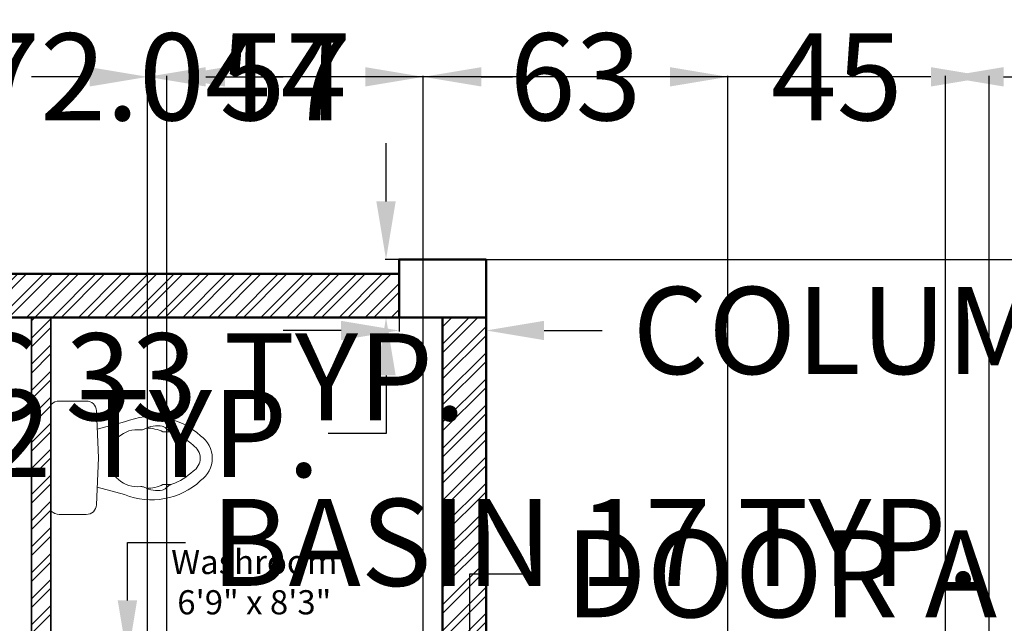
# Model space of a CAD drawing. Units: inches. Extents: x -90 to 536, y -553 to 299.
# Tile 26 of 27: x 207 to 410, y 174 to 299. Entities that reach past the tile are written whole.
import ezdxf

# ---------------------------------------------------------------- set-up
doc = ezdxf.new("R2010")
doc.units = ezdxf.units.IN
for name, color, linetype, lineweight in [('A-ANNO-DIMS', 2, 'Continuous', 18), ('A-AREA-IDEN', 7, 'Continuous', 18), ('A-COLS', 7, 'Continuous', 50), ('A-FLOR-FIXT', 8, 'Continuous', 18), ('A-WALL-PATT', 252, 'Continuous', 13), ('Inner Wall', 5, 'Continuous', 35), ('Outer Wall', 1, 'Continuous', 50)]:
    doc.layers.add(name, color=color, linetype=linetype, lineweight=lineweight)
doc.styles.get("Standard").update_dxf_attribs({"font": 'arial.ttf'})
doc.dimstyles.get("Standard").update_dxf_attribs({"dimtxt": 18, "dimasz": 12, "dimexe": 0.18, "dimexo": 0.0625, "dimgap": 0.09, "dimtad": 0, "dimtih": 1, "dimtoh": 1, "dimdec": 0, "dimzin": 0, "dimdsep": 46, "dimlunit": 3, "dimtxsty": 'Standard', "dimcen": 0.09, "dimadec": 0, "dimazin": 0, "dimtfac": 1, "dimtdec": 0, "dimtofl": 0, "dimtmove": 0, "dimatfit": 3, "dimfxl": 1, "dimtolj": 1, "dimtzin": 0, "dimarcsym": 0})

# ---------------------------------------------------------------- blocks, each defined once
blk = doc.blocks.new('A$C1308471B')
at = {"ltscale": 20}
for p, q in [((0, 0.4607), (0, 0.0186)), ((0.0354, 0.4793), (0.1495, 0.4793)), ((0.2013, 0.2397), (0.1923, 0.4384)), ((0.1957, 0.3639), (0.3109, 0.3953)), ((0.5021, 0.3528), (0.4724, 0.3528)), ((0.4982, 0.3575), (0.4822, 0.3709)), ((0.2013, 0.2397), (0.1923, 0.0409)), ((0.5021, 0.1304), (0.4724, 0.1304)), ((0.4982, 0.1257), (0.4822, 0.1123)), ((0.1959, 0.1193), (0.3109, 0.0879)), ((0.0354, 0), (0.1495, 0))]:
    blk.add_line(p, q, dxfattribs=at)
for centre, radius, start, end in [((0.006, 0.4607), 0.006, 136.5269, 180), ((0.0354, 0.4328), 0.0465, 90, 136.5269), ((0.1495, 0.4365), 0.0429, 2.5755, 90), ((0.4248, 0.1104), 0.3068, 47.4135, 111.7924), ((0.4494, 0.2636), 0.1148, 79.3968, 118.5742), ((0.4658, 0.3513), 0.0255, 50, 79.3968), ((0.3654, 0.2416), 0.1206, 83.3523, 180), ((0.3823, 0.3868), 0.0255, 263.3523, 298.5742), ((0.405, 0.2159), 0.153, 63.502, 90.4522), ((0.5146, 0.377), 0.0255, 230, 251.3881), ((0.5021, 0.3273), 0.0255, 70.3751, 90), ((0.4248, 0.1104), 0.2558, 46.612, 70.3751), ((0.5654, 0.2416), 0.116, 0, 54.7115), ((0.5654, 0.2416), 0.065, 0, 57.2974), ((0.3654, 0.2416), 0.1206, 180, 276.6477), ((0.5654, 0.2416), 0.065, 302.7026, 0), ((0.5654, 0.2416), 0.116, 305.2885, 0), ((0.4248, 0.3728), 0.2558, 289.6249, 313.388), ((0.4248, 0.3728), 0.3068, 248.2076, 312.5865), ((0.405, 0.2673), 0.153, 269.5478, 296.498), ((0.5146, 0.1062), 0.0255, 108.6119, 130), ((0.5021, 0.1559), 0.0255, 270, 289.6249), ((0.3823, 0.0964), 0.0255, 61.4258, 96.6477), ((0.4494, 0.2196), 0.1148, 241.4258, 280.6032), ((0.4658, 0.1319), 0.0255, 280.6032, 310), ((0.006, 0.0186), 0.006, 180, 223.4731), ((0.0354, 0.0465), 0.0465, 223.4731, 270), ((0.1495, 0.0429), 0.0429, 270, 357.4245)]:
    blk.add_arc(centre, radius, start, end, dxfattribs=at)
blk = doc.blocks.new('COL-12X18')
blk.add_lwpolyline([(0, 18), (12, 18), (12, 0), (0, 0)], close=True)
blk = doc.blocks.new('*D19')
at = {"layer": 'A-ANNO-DIMS', "color": 0, "lineweight": -2, "transparency": 16777216}
for p, q in [((299.76, 172.45), (299.76, 184.45)), ((299.76, 184.45), (311.76, 184.45)), ((294.19, 172.45), (299.94, 172.45)), ((299.76, 146.95), (299.76, 160.45)), ((294.19, 134.95), (299.94, 134.95))]:
    blk.add_line(p, q, dxfattribs=at)
at = {"layer": 'A-ANNO-DIMS', "color": 0, "transparency": 16777216}
for points in [[(297.76, 160.45), (301.76, 160.45), (299.76, 172.45)], [(297.76, 146.95), (301.76, 146.95), (299.76, 134.95)]]:
    blk.add_solid(points, dxfattribs=at)
at = {"layer": 'Defpoints', "color": 0, "transparency": 16777216}
for p in [(294.13, 172.45), (299.76, 172.45), (294.13, 134.95)]:
    blk.add_point(p, dxfattribs=at)
at = {"layer": 'A-ANNO-DIMS', "color": 0, "transparency": 16777216, "insert": (408.3, 184.45), "char_height": 18, "attachment_point": 5}
blk.add_mtext('\\A1;DOOR A 38 TYP.', dxfattribs=at)
blk = doc.blocks.new('*D21')
at = {"layer": 'A-ANNO-DIMS', "color": 0, "lineweight": -2, "transparency": 16777216}
for p, q in [((122.13, 220.23), (122.13, 225.35)), ((134.13, 225.17), (143.49, 225.17)), ((155.49, 220.23), (155.49, 225.35)), ((155.49, 225.17), (167.49, 225.17))]:
    blk.add_line(p, q, dxfattribs=at)
at = {"layer": 'A-ANNO-DIMS', "color": 0, "transparency": 16777216}
for points in [[(134.13, 227.17), (134.13, 223.17), (122.13, 225.17)], [(143.49, 227.17), (143.49, 223.17), (155.49, 225.17)]]:
    blk.add_solid(points, dxfattribs=at)
at = {"layer": 'Defpoints', "color": 0, "transparency": 16777216}
for p in [(155.49, 225.17), (122.13, 220.17), (155.49, 220.17)]:
    blk.add_point(p, dxfattribs=at)
at = {"layer": 'A-ANNO-DIMS', "color": 0, "transparency": 16777216, "insert": (236.2, 225.17), "char_height": 18, "attachment_point": 5}
blk.add_mtext('\\A1;WC 33 TYP.', dxfattribs=at)
blk = doc.blocks.new('*D23')
at = {"layer": 'A-ANNO-DIMS', "color": 0, "lineweight": -2, "transparency": 16777216}
for p, q in [((285.13, 237.38), (285.13, 234.57)), ((303.13, 237.38), (303.13, 234.57)), ((273.13, 234.75), (261.13, 234.75)), ((315.13, 234.75), (327.13, 234.75))]:
    blk.add_line(p, q, dxfattribs=at)
at = {"layer": 'A-ANNO-DIMS', "color": 0, "transparency": 16777216}
for points in [[(273.13, 236.75), (273.13, 232.75), (285.13, 234.75)], [(315.13, 236.75), (315.13, 232.75), (303.13, 234.75)]]:
    blk.add_solid(points, dxfattribs=at)
at = {"layer": 'Defpoints', "color": 0, "transparency": 16777216}
for p in [(285.13, 237.45), (303.13, 237.45), (303.13, 234.75)]:
    blk.add_point(p, dxfattribs=at)
at = {"layer": 'A-ANNO-DIMS', "color": 0, "transparency": 16777216, "insert": (428.9, 234.75), "char_height": 18, "attachment_point": 5}
blk.add_mtext('\\A1;COLUMN 18 TYP.', dxfattribs=at)
blk = doc.blocks.new('*D24')
at = {"layer": 'A-ANNO-DIMS', "color": 0, "lineweight": -2, "transparency": 16777216}
for p, q in [((282.43, 261.45), (282.43, 273.45)), ((285.07, 249.45), (282.25, 249.45)), ((285.07, 237.45), (282.25, 237.45)), ((282.43, 225.45), (282.43, 213.45)), ((282.43, 213.45), (270.43, 213.45))]:
    blk.add_line(p, q, dxfattribs=at)
at = {"layer": 'A-ANNO-DIMS', "color": 0, "transparency": 16777216}
for points in [[(280.43, 261.45), (284.43, 261.45), (282.43, 249.45)], [(280.43, 225.45), (284.43, 225.45), (282.43, 237.45)]]:
    blk.add_solid(points, dxfattribs=at)
at = {"layer": 'Defpoints', "color": 0, "transparency": 16777216}
for p in [(285.13, 249.45), (282.43, 237.45), (285.13, 237.45)]:
    blk.add_point(p, dxfattribs=at)
at = {"layer": 'A-ANNO-DIMS', "color": 0, "transparency": 16777216, "insert": (227.38, 213.45), "char_height": 18, "attachment_point": 5}
blk.add_mtext('\\A1;12 TYP.', dxfattribs=at)
blk = doc.blocks.new('*D25')
at = {"layer": 'A-ANNO-DIMS', "color": 0, "lineweight": -2, "transparency": 16777216}
for p, q in [((228.95, 178.94), (228.95, 190.94)), ((228.95, 190.94), (240.95, 190.94)), ((226.49, 166.94), (229.13, 166.94)), ((226.49, 150.15), (229.13, 150.15)), ((228.95, 138.15), (228.95, 126.15))]:
    blk.add_line(p, q, dxfattribs=at)
at = {"layer": 'A-ANNO-DIMS', "color": 0, "transparency": 16777216}
for points in [[(226.95, 178.94), (230.95, 178.94), (228.95, 166.94)], [(226.95, 138.15), (230.95, 138.15), (228.95, 150.15)]]:
    blk.add_solid(points, dxfattribs=at)
at = {"layer": 'Defpoints', "color": 0, "transparency": 16777216}
for p in [(226.43, 166.94), (228.95, 166.94), (226.43, 150.15)]:
    blk.add_point(p, dxfattribs=at)
at = {"layer": 'A-ANNO-DIMS', "color": 0, "transparency": 16777216, "insert": (325.67, 190.94), "char_height": 18, "attachment_point": 5}
blk.add_mtext('\\A1;BASIN 17 TYP.', dxfattribs=at)
blk = doc.blocks.new('*D26')
at = {"layer": 'A-ANNO-DIMS', "color": 0, "lineweight": -2, "transparency": 16777216}
for p, q in [((201.13, 169.45), (189.13, 169.45)), ((213.13, 167), (213.13, 169.63)), ((226.43, 167), (226.43, 169.63)), ((238.43, 169.45), (250.43, 169.45))]:
    blk.add_line(p, q, dxfattribs=at)
at = {"layer": 'A-ANNO-DIMS', "color": 0, "transparency": 16777216}
for points in [[(201.13, 171.45), (201.13, 167.45), (213.13, 169.45)], [(238.43, 171.45), (238.43, 167.45), (226.43, 169.45)]]:
    blk.add_solid(points, dxfattribs=at)
at = {"layer": 'Defpoints', "color": 0, "transparency": 16777216}
for p in [(213.13, 169.45), (213.13, 166.94), (226.43, 166.94)]:
    blk.add_point(p, dxfattribs=at)
at = {"layer": 'A-ANNO-DIMS', "color": 0, "transparency": 16777216, "insert": (146.08, 169.45), "char_height": 18, "attachment_point": 5}
blk.add_mtext('\\A1;13 TYP.', dxfattribs=at)
blk = doc.blocks.new('*D53')
at = {"layer": 'A-ANNO-DIMS', "color": 0, "lineweight": -2, "transparency": 16777216}
for p, q in [((35.09, 103.75), (35.09, 287.38)), ((47.09, 287.2), (183.7, 287.2)), ((395.13, 287.2), (258.52, 287.2)), ((407.13, -63.49), (407.13, 287.38))]:
    blk.add_line(p, q, dxfattribs=at)
at = {"layer": 'A-ANNO-DIMS', "color": 0, "transparency": 16777216}
for points in [[(47.09, 289.2), (47.09, 285.2), (35.09, 287.2)], [(395.13, 289.2), (395.13, 285.2), (407.13, 287.2)]]:
    blk.add_solid(points, dxfattribs=at)
at = {"layer": 'Defpoints', "color": 0, "transparency": 16777216}
for p in [(407.13, 287.2), (35.09, 103.69), (407.13, -63.55)]:
    blk.add_point(p, dxfattribs=at)
at = {"layer": 'A-ANNO-DIMS', "color": 0, "transparency": 16777216, "insert": (221.11, 287.2), "char_height": 18, "attachment_point": 5}
blk.add_mtext('\\A1;372.04', dxfattribs=at)
blk = doc.blocks.new('*D58')
at = {"layer": 'A-ANNO-DIMS', "color": 0, "lineweight": -2, "transparency": 16777216}
for p, q in [((290.13, -71.49), (290.13, 287.38)), ((302.13, 287.2), (308.6, 287.2)), ((341.13, 287.2), (334.66, 287.2)), ((353.13, -71.49), (353.13, 287.38))]:
    blk.add_line(p, q, dxfattribs=at)
at = {"layer": 'A-ANNO-DIMS', "color": 0, "transparency": 16777216}
for points in [[(302.13, 289.2), (302.13, 285.2), (290.13, 287.2)], [(341.13, 289.2), (341.13, 285.2), (353.13, 287.2)]]:
    blk.add_solid(points, dxfattribs=at)
at = {"layer": 'Defpoints', "color": 0, "transparency": 16777216}
for p in [(353.13, 287.2), (290.13, -71.55), (353.13, -71.55)]:
    blk.add_point(p, dxfattribs=at)
at = {"layer": 'A-ANNO-DIMS', "color": 0, "transparency": 16777216, "insert": (321.63, 287.2), "char_height": 18, "attachment_point": 5}
blk.add_mtext('\\A1;63', dxfattribs=at)
blk = doc.blocks.new('*D59')
at = {"layer": 'A-ANNO-DIMS', "color": 0, "lineweight": -2, "transparency": 16777216}
for p, q in [((341.13174, 287.201217), (329.13174, 287.201217)), ((353.13174, -71.491283), (353.13174, 287.381217)), ((398.13174, -71.491283), (398.13174, 287.381217)), ((410.13174, 287.201217), (422.13174, 287.201217))]:
    blk.add_line(p, q, dxfattribs=at)
at = {"layer": 'A-ANNO-DIMS', "color": 0, "transparency": 16777216}
for points in [[(341.13174, 289.201217), (341.13174, 285.201217), (353.13174, 287.201217)], [(410.13174, 289.201217), (410.13174, 285.201217), (398.13174, 287.201217)]]:
    blk.add_solid(points, dxfattribs=at)
at = {"layer": 'Defpoints', "color": 0, "transparency": 16777216}
for p in [(398.13174, 287.201217), (353.13174, -71.553783), (398.13174, -71.553783)]:
    blk.add_point(p, dxfattribs=at)
at = {"layer": 'A-ANNO-DIMS', "color": 0, "transparency": 16777216, "insert": (375.63174, 287.201217), "char_height": 18, "attachment_point": 5}
blk.add_mtext('\\A1;45', dxfattribs=at)
blk = doc.blocks.new('*D62')
at = {"layer": 'A-ANNO-DIMS', "color": 0, "lineweight": -2, "transparency": 16777216}
for p, q in [((233.13, -71.49), (233.13, 287.38)), ((245.13, 287.2), (248.65, 287.2)), ((278.13, 287.2), (274.61, 287.2)), ((290.13, -71.49), (290.13, 287.38))]:
    blk.add_line(p, q, dxfattribs=at)
at = {"layer": 'A-ANNO-DIMS', "color": 0, "transparency": 16777216}
for points in [[(245.13, 289.2), (245.13, 285.2), (233.13, 287.2)], [(278.13, 289.2), (278.13, 285.2), (290.13, 287.2)]]:
    blk.add_solid(points, dxfattribs=at)
at = {"layer": 'Defpoints', "color": 0, "transparency": 16777216}
for p in [(290.13, 287.2), (233.13, -71.55), (290.13, -71.55)]:
    blk.add_point(p, dxfattribs=at)
at = {"layer": 'A-ANNO-DIMS', "color": 0, "transparency": 16777216, "insert": (261.63, 287.2), "char_height": 18, "attachment_point": 5}
blk.add_mtext('\\A1;57', dxfattribs=at)
blk = doc.blocks.new('*D65')
at = {"layer": 'A-ANNO-DIMS', "color": 0, "lineweight": -2, "transparency": 16777216}
for p, q in [((221.13, 287.2), (209.13, 287.2)), ((233.13, 134.51), (233.13, 287.38)), ((237.13, 134.51), (237.13, 287.38)), ((249.13, 287.2), (261.13, 287.2))]:
    blk.add_line(p, q, dxfattribs=at)
at = {"layer": 'A-ANNO-DIMS', "color": 0, "transparency": 16777216}
for points in [[(221.13, 289.2), (221.13, 285.2), (233.13, 287.2)], [(249.13, 289.2), (249.13, 285.2), (237.13, 287.2)]]:
    blk.add_solid(points, dxfattribs=at)
at = {"layer": 'Defpoints', "color": 0, "transparency": 16777216}
for p in [(237.13, 287.2), (233.13, 134.45), (237.13, 134.45)]:
    blk.add_point(p, dxfattribs=at)
at = {"layer": 'A-ANNO-DIMS', "color": 0, "transparency": 16777216, "insert": (267.45, 287.2), "char_height": 18, "attachment_point": 5}
blk.add_mtext('\\A1;4', dxfattribs=at)
blk = doc.blocks.new('*D66')
at = {"layer": 'A-ANNO-DIMS', "color": 0, "lineweight": -2, "transparency": 16777216}
for p, q in [((303.19, 249.45), (445.07, 249.45)), ((444.89, 237.45), (444.89, 205.73)), ((444.89, 155.45), (444.89, 187.17)), ((381.19, 143.45), (445.07, 143.45))]:
    blk.add_line(p, q, dxfattribs=at)
at = {"layer": 'A-ANNO-DIMS', "color": 0, "transparency": 16777216}
for points in [[(442.89, 237.45), (446.89, 237.45), (444.89, 249.45)], [(442.89, 155.45), (446.89, 155.45), (444.89, 143.45)]]:
    blk.add_solid(points, dxfattribs=at)
at = {"layer": 'Defpoints', "color": 0, "transparency": 16777216}
for p in [(303.13, 249.45), (444.89, 249.45), (381.13, 143.45)]:
    blk.add_point(p, dxfattribs=at)
at = {"layer": 'A-ANNO-DIMS', "color": 0, "transparency": 16777216, "insert": (444.89, 196.45), "char_height": 18, "attachment_point": 5}
blk.add_mtext('\\A1;106', dxfattribs=at)

msp = doc.modelspace()

# ---------------------------------------------------------------- hatches: boundary and pattern name
at = {"layer": 'A-WALL-PATT'}
h = msp.add_hatch(dxfattribs=at)
h.set_pattern_fill('ANSI32', color=256, scale=0.4)
h.set_pattern_definition([(45, (-88.8105, -603.6155), (-2.694077, 2.694077), []), (45, (-87.0145, -603.6155), (-2.694077, 2.694077), [])])
h.paths.add_polyline_path([(285.1317, 246.4462), (131.1317, 246.4462), (131.1317, 237.4462), (285.1317, 237.4462)])
h.paths.add_polyline_path([(122.1317, 237.4462), (113.1317, 237.4462), (113.1317, 152.4462), (122.1317, 152.4462), (122.1317, 166.4704)])
h.paths.add_polyline_path([(303.1317, 237.4462), (294.1317, 237.4462), (294.1317, 152.4462), (303.1317, 152.4462)])
h.paths.add_polyline_path([(47.1317, 91.9277), (38.1317, 91.9277), (38.1317, -6.5538), (77.1317, -6.5538), (77.1317, 2.4462), (70.5655, 2.4462), (47.1317, 2.4462)])
h.paths.add_polyline_path([(83.052, -61.5538), (47.1317, -61.5538), (47.1317, -24.5538), (38.1317, -24.5538), (38.1317, -70.5538), (74.052, -70.5538), (74.052, -223.5538), (38.1317, -223.5538), (38.1317, -503.5538), (92.1317, -503.5538), (92.1317, -437.5538), (191.1317, -437.5538), (191.1317, -428.5538), (83.1317, -428.5538), (83.1317, -494.5538), (47.1317, -494.5538), (47.1317, -232.5538), (83.052, -232.5538), (83.052, -70.5538)])
h.paths.add_polyline_path([(407.1317, -63.5538), (381.1317, -63.5538), (381.1317, 91.9277), (372.1317, 91.9277), (372.1317, 32.8805), (372.1317, -63.5538), (306.5745, -63.5538), (237.1317, -63.5538), (237.1317, -38.5538), (233.1317, -38.5538), (233.1317, -71.5538), (398.1317, -71.5538), (398.1317, -152.5538), (233.1317, -152.5538), (233.1317, -161.5538), (398.1317, -161.5538), (398.1317, -368.5538), (233.1317, -368.5538), (233.1317, -377.5538), (407.1317, -377.5538), (407.1317, -161.5538)])
h.paths.add_polyline_path([(261.1317, -422.5538), (252.1317, -422.5538), (252.1317, -428.5538), (233.1317, -428.5538), (233.1317, -437.5538), (261.1317, -437.5538)])
h.paths.add_polyline_path([(191.1317, -368.5538), (180.1317, -368.5538), (180.1317, -335.5538), (131.5919, -335.5538), (131.5919, -344.5538), (171.1317, -344.5538), (171.1317, -392.5538), (180.1317, -392.5538), (180.1317, -377.5538), (191.1317, -377.5538)], flags=17)
h.paths.add_polyline_path([(180.1317, -223.5538), (152.1317, -223.5538), (152.1317, -227.5538), (176.1317, -227.5538), (176.1317, -335.5538), (180.1317, -335.5538)], flags=17)
h.paths.add_polyline_path([(131.5919, -335.5538), (83.1317, -335.5538), (83.1317, -339.5538), (83.1317, -392.5538), (87.1317, -392.5538), (87.1317, -339.5538), (131.5919, -339.5538)], flags=17)
h.paths.add_polyline_path([(197.1317, 2.4462), (77.1317, 2.4462), (77.1317, -1.5538), (113.1317, -1.5538), (113.1317, -71.5538), (181.1317, -71.5538), (181.1317, -67.5538), (117.1317, -67.5538), (117.1317, -1.5538), (177.1317, -1.5538), (177.1317, -37.5538), (181.1317, -37.5538), (181.1317, -1.5538), (197.1317, -1.5538)])
h.paths.add_polyline_path([(173.1317, 138.4462), (122.1317, 138.4462), (122.1317, 134.4462), (173.1317, 134.4462)])
h.paths.add_polyline_path([(213.1317, 237.4462), (209.1317, 237.4462), (209.1317, 134.4462), (233.1317, 134.4462), (233.1317, 68.8889), (233.1317, -2.5538), (237.1317, -2.5538), (237.1317, 134.4462), (258.1317, 134.4462), (258.1317, 138.4462), (213.1317, 138.4462)])

# ---------------------------------------------------------------- linework, layer by layer
at = {"layer": 'Inner Wall'}
for p, q in [((209.1317, 237.4462), (209.1317, 134.4462)), ((213.1317, 237.4462), (213.1317, 138.4462))]:
    msp.add_line(p, q, dxfattribs=at)
at = {"layer": 'Outer Wall'}
for p, q in [((131.1317, 246.4462), (285.1317, 246.4462)), ((303.1317, 246.4462), (303.1317, 152.4462)), ((122.1317, 237.4462), (294.1317, 237.4462)), ((294.1317, 237.4462), (294.1317, 134.4462))]:
    msp.add_line(p, q, dxfattribs=at)

# ---------------------------------------------------------------- block references
at = {"layer": 'A-COLS', "rotation": 270.0000000000002}
msp.add_blockref('COL-12X18', (285.1317, 249.4462), dxfattribs=at)
at = {"layer": 'A-FLOR-FIXT', "xscale": -48.95497407897215, "yscale": 48.95497407897215, "zscale": 48.95497407897215, "rotation": 180}
msp.add_blockref('A$C1308471B', (213.1317, 220.1654), dxfattribs=at)

# ---------------------------------------------------------------- texts
at = {"layer": 'A-AREA-IDEN', "insert": (272.803, 189.3861), "char_height": 5, "attachment_point": 3}
msp.add_mtext_dynamic_manual_height_columns('\\pxqc;{\\fTimes New Roman|b0|i0|c0|p18;Washroom\\P6\'9" x 8\'3"}', width=35.23368, gutter_width=12.5, heights=[0], dxfattribs=at)

# ---------------------------------------------------------------- dimensions: what is measured, and where the dimension line sits
at = {"layer": 'A-ANNO-DIMS'}
for base, p1, p2, override, picture, middle in [((407.1317, 287.2012), (35.0873, 103.6916), (407.1317, -63.5538), {"dimdec": 2, "dimlfac": 1, "dimrnd": 0, "dimzin": 0, "dimdsep": 46, "dimlunit": 2}, '*D53', (221.1095, 287.2012)), ((237.1317, 287.2012), (233.1317, 134.4462), (237.1317, 134.4462), {"dimdec": 0, "dimlfac": 1, "dimrnd": 0, "dimzin": 0, "dimdsep": 46, "dimlunit": 2}, '*D65', (267.4468, 287.2012)), ((290.1317, 287.2012), (233.1317, -71.5538), (290.1317, -71.5538), {"dimdec": 0, "dimlfac": 1, "dimrnd": 0, "dimzin": 0, "dimdsep": 46, "dimlunit": 2}, '*D62', (261.6317, 287.2012)), ((353.1317, 287.2012), (290.1317, -71.5538), (353.1317, -71.5538), {"dimdec": 0, "dimlfac": 1, "dimrnd": 0, "dimzin": 0, "dimdsep": 46, "dimlunit": 2}, '*D58', (321.6317, 287.2012)), ((398.1317, 287.2012), (353.1317, -71.5538), (398.1317, -71.5538), {"dimdec": 0, "dimlfac": 1, "dimrnd": 0, "dimzin": 0, "dimdsep": 46, "dimlunit": 2}, '*D59', (375.6317, 287.2012))]:
    dim = msp.add_linear_dim(base=base, p1=p1, p2=p2, dimstyle='Standard', override=override, dxfattribs=at)
    dim.commit()
    dim.dimension.update_dxf_attribs({"geometry": picture, "text_midpoint": middle})
for base, p1, p2, angle, text, picture, middle in [((303.1317, 234.7462), (285.1317, 237.4462), (303.1317, 237.4462), 0, 'COLUMN <> TYP.', '*D23', (428.9046, 234.7462)), ((282.4317, 237.4462), (285.1317, 249.4462), (285.1317, 237.4462), 270, '<> TYP.', '*D24', (227.3799, 213.4462)), ((299.7567404714, 172.4462174295), (294.1317404714, 134.9462174295), (294.1317404714, 172.4462174295), 90, 'DOOR A <> TYP.', '*D19', (408.2989914946, 184.4462174295)), ((228.949, 166.9352), (226.4312, 150.1495), (226.4312, 166.9352), 90, 'BASIN <> TYP.', '*D25', (325.6734, 190.9352)), ((213.1317, 169.4531), (226.4312, 166.9352), (213.1317, 166.9352), 180, '<> TYP.', '*D26', (146.0799, 169.4531))]:
    dim = msp.add_linear_dim(base=base, p1=p1, p2=p2, angle=angle, text=text, dimstyle='Standard', override={"dimdec": 0, "dimlfac": 1, "dimrnd": 0, "dimzin": 0, "dimdsep": 46, "dimlunit": 2}, dxfattribs=at)
    dim.commit()
    dim.dimension.update_dxf_attribs({"geometry": picture, "text_midpoint": middle})
dim = msp.add_linear_dim(base=(155.4885, 225.1689), p1=(122.1317, 220.1654), p2=(155.4885, 220.1654), text='WC <> TYP.', dimstyle='Standard', override={"dimdec": 0, "dimlfac": 1, "dimrnd": 0, "dimzin": 0, "dimdsep": 46, "dimlunit": 2}, dxfattribs=at)
dim.commit()
dim.dimension.update_dxf_attribs({"geometry": '*D21', "text_midpoint": (236.1958, 225.1689)})
dim = msp.add_linear_dim(base=(444.8867, 249.4462), p1=(381.1317, 143.4462), p2=(303.1317, 249.4462), angle=90, dimstyle='Standard', override={"dimdec": 0, "dimlfac": 1, "dimrnd": 0, "dimzin": 0, "dimdsep": 46, "dimlunit": 2}, dxfattribs=at)
dim.commit()
dim.dimension.update_dxf_attribs({"geometry": '*D66', "text_midpoint": (444.8867, 196.4462)})

doc.saveas('drawing.dxf')
